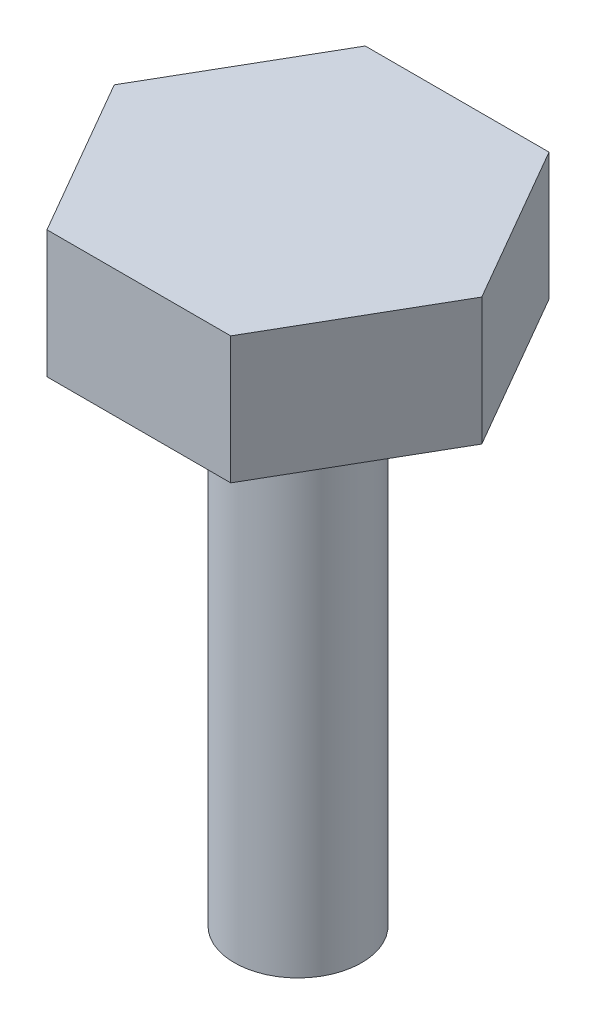
ISO-10303-21;
HEADER;
FILE_DESCRIPTION(('STEP AP214'),'2;1');
FILE_NAME('part.step','',(''),(''),'','','');
FILE_SCHEMA(('AUTOMOTIVE_DESIGN { 1 0 10303 214 1 1 1 1 }'));
ENDSEC;
DATA;
#1=APPLICATION_CONTEXT('core data for automotive mechanical design processes');
#2=APPLICATION_PROTOCOL_DEFINITION('international standard','automotive_design',2000,#1);
#3=PRODUCT_CONTEXT('',#1,'mechanical');
#4=PRODUCT('Part','Part','',(#3));
#5=PRODUCT_RELATED_PRODUCT_CATEGORY('part','',(#4));
#6=PRODUCT_DEFINITION_FORMATION('','',#4);
#7=PRODUCT_DEFINITION_CONTEXT('part definition',#1,'design');
#8=PRODUCT_DEFINITION('design','',#6,#7);
#9=PRODUCT_DEFINITION_SHAPE('','',#8);
#10=(LENGTH_UNIT() NAMED_UNIT(*) SI_UNIT(.MILLI.,.METRE.));
#11=(NAMED_UNIT(*) PLANE_ANGLE_UNIT() SI_UNIT($,.RADIAN.));
#12=(NAMED_UNIT(*) SI_UNIT($,.STERADIAN.) SOLID_ANGLE_UNIT());
#13=UNCERTAINTY_MEASURE_WITH_UNIT(LENGTH_MEASURE(1.E-05),#10,'distance_accuracy_value','');
#14=(GEOMETRIC_REPRESENTATION_CONTEXT(3) GLOBAL_UNCERTAINTY_ASSIGNED_CONTEXT((#13)) GLOBAL_UNIT_ASSIGNED_CONTEXT((#10,
#11,#12)) REPRESENTATION_CONTEXT('',''));
#15=CARTESIAN_POINT('',(0.,0.,0.));
#16=DIRECTION('',(0.,0.,1.));
#17=DIRECTION('',(1.,0.,0.));
#18=AXIS2_PLACEMENT_3D('',#15,#16,#17);
#19=CARTESIAN_POINT('',(14.4337567297409,20.,24.9999999999998));
#20=DIRECTION('',(-0.866025403784442,0.,-0.499999999999995));
#21=DIRECTION('',(-0.499999999999995,0.,0.866025403784442));
#22=AXIS2_PLACEMENT_3D('',#19,#20,#21);
#23=PLANE('',#22);
#24=DIRECTION('',(0.499999999999995,0.,-0.866025403784441));
#25=VECTOR('',#24,1.);
#26=CARTESIAN_POINT('',(14.4337567297409,0.,24.9999999999998));
#27=LINE('',#26,#25);
#28=CARTESIAN_POINT('',(14.4337567297409,0.,24.9999999999998));
#29=VERTEX_POINT('',#28);
#30=CARTESIAN_POINT('',(28.8675134594813,0.,0.));
#31=VERTEX_POINT('',#30);
#32=EDGE_CURVE('E124',#29,#31,#27,.T.);
#33=ORIENTED_EDGE('',*,*,#32,.T.);
#34=DIRECTION('',(0.,-1.,0.));
#35=VECTOR('',#34,1.);
#36=CARTESIAN_POINT('',(28.8675134594813,20.,0.));
#37=LINE('',#36,#35);
#38=CARTESIAN_POINT('',(28.8675134594813,20.,0.));
#39=VERTEX_POINT('',#38);
#40=EDGE_CURVE('E45',#39,#31,#37,.T.);
#41=ORIENTED_EDGE('',*,*,#40,.F.);
#42=DIRECTION('',(0.499999999999995,0.,-0.866025403784441));
#43=VECTOR('',#42,1.);
#44=CARTESIAN_POINT('',(14.4337567297409,20.,24.9999999999998));
#45=LINE('',#44,#43);
#46=CARTESIAN_POINT('',(14.4337567297409,20.,24.9999999999998));
#47=VERTEX_POINT('',#46);
#48=EDGE_CURVE('E138',#47,#39,#45,.T.);
#49=ORIENTED_EDGE('',*,*,#48,.F.);
#50=DIRECTION('',(0.,-1.,0.));
#51=VECTOR('',#50,1.);
#52=CARTESIAN_POINT('',(14.4337567297409,20.,24.9999999999998));
#53=LINE('',#52,#51);
#54=EDGE_CURVE('E123',#47,#29,#53,.T.);
#55=ORIENTED_EDGE('',*,*,#54,.T.);
#56=EDGE_LOOP('',(#33,#41,#49,#55));
#57=FACE_BOUND('',#56,.T.);
#58=ADVANCED_FACE('F39',(#57),#23,.F.);
#59=CARTESIAN_POINT('',(28.8675134594813,20.,0.));
#60=DIRECTION('',(-0.866025403784438,0.,0.500000000000001));
#61=DIRECTION('',(0.500000000000001,0.,0.866025403784438));
#62=AXIS2_PLACEMENT_3D('',#59,#60,#61);
#63=PLANE('',#62);
#64=DIRECTION('',(-0.500000000000001,0.,-0.866025403784438));
#65=VECTOR('',#64,1.);
#66=CARTESIAN_POINT('',(28.8675134594813,0.,0.));
#67=LINE('',#66,#65);
#68=CARTESIAN_POINT('',(14.4337567297406,0.,-25.0000000000001));
#69=VERTEX_POINT('',#68);
#70=EDGE_CURVE('E126',#31,#69,#67,.T.);
#71=ORIENTED_EDGE('',*,*,#70,.T.);
#72=DIRECTION('',(0.,-1.,0.));
#73=VECTOR('',#72,1.);
#74=CARTESIAN_POINT('',(14.4337567297406,20.,-25.0000000000001));
#75=LINE('',#74,#73);
#76=CARTESIAN_POINT('',(14.4337567297406,20.,-25.0000000000001));
#77=VERTEX_POINT('',#76);
#78=EDGE_CURVE('E137',#77,#69,#75,.T.);
#79=ORIENTED_EDGE('',*,*,#78,.F.);
#80=DIRECTION('',(-0.500000000000001,0.,-0.866025403784438));
#81=VECTOR('',#80,1.);
#82=CARTESIAN_POINT('',(28.8675134594813,20.,0.));
#83=LINE('',#82,#81);
#84=EDGE_CURVE('E94',#39,#77,#83,.T.);
#85=ORIENTED_EDGE('',*,*,#84,.F.);
#86=ORIENTED_EDGE('',*,*,#40,.T.);
#87=EDGE_LOOP('',(#71,#79,#85,#86));
#88=FACE_BOUND('',#87,.T.);
#89=ADVANCED_FACE('F145',(#88),#63,.F.);
#90=CARTESIAN_POINT('',(14.4337567297406,20.,-25.0000000000001));
#91=DIRECTION('',(0.,0.,1.));
#92=DIRECTION('',(1.,0.,0.));
#93=AXIS2_PLACEMENT_3D('',#90,#91,#92);
#94=PLANE('',#93);
#95=DIRECTION('',(-1.,0.,0.));
#96=VECTOR('',#95,1.);
#97=CARTESIAN_POINT('',(14.4337567297406,0.,-25.0000000000001));
#98=LINE('',#97,#96);
#99=CARTESIAN_POINT('',(-14.4337567297408,0.,-25.));
#100=VERTEX_POINT('',#99);
#101=EDGE_CURVE('E133',#69,#100,#98,.T.);
#102=ORIENTED_EDGE('',*,*,#101,.T.);
#103=DIRECTION('',(0.,-1.,0.));
#104=VECTOR('',#103,1.);
#105=CARTESIAN_POINT('',(-14.4337567297408,20.,-25.));
#106=LINE('',#105,#104);
#107=CARTESIAN_POINT('',(-14.4337567297408,20.,-25.));
#108=VERTEX_POINT('',#107);
#109=EDGE_CURVE('E118',#108,#100,#106,.T.);
#110=ORIENTED_EDGE('',*,*,#109,.F.);
#111=DIRECTION('',(-1.,0.,0.));
#112=VECTOR('',#111,1.);
#113=CARTESIAN_POINT('',(14.4337567297406,20.,-25.0000000000001));
#114=LINE('',#113,#112);
#115=EDGE_CURVE('E110',#77,#108,#114,.T.);
#116=ORIENTED_EDGE('',*,*,#115,.F.);
#117=ORIENTED_EDGE('',*,*,#78,.T.);
#118=EDGE_LOOP('',(#102,#110,#116,#117));
#119=FACE_BOUND('',#118,.T.);
#120=ADVANCED_FACE('F147',(#119),#94,.F.);
#121=CARTESIAN_POINT('',(-14.4337567297408,20.,-25.));
#122=DIRECTION('',(0.866025403784442,0.,0.499999999999995));
#123=DIRECTION('',(0.499999999999995,0.,-0.866025403784442));
#124=AXIS2_PLACEMENT_3D('',#121,#122,#123);
#125=PLANE('',#124);
#126=DIRECTION('',(-0.499999999999995,0.,0.866025403784442));
#127=VECTOR('',#126,1.);
#128=CARTESIAN_POINT('',(-14.4337567297408,0.,-25.));
#129=LINE('',#128,#127);
#130=CARTESIAN_POINT('',(-28.8675134594813,0.,2.01580769085164E-13));
#131=VERTEX_POINT('',#130);
#132=EDGE_CURVE('E113',#100,#131,#129,.T.);
#133=ORIENTED_EDGE('',*,*,#132,.T.);
#134=DIRECTION('',(0.,-1.,0.));
#135=VECTOR('',#134,1.);
#136=CARTESIAN_POINT('',(-28.8675134594813,20.,2.01580769085164E-13));
#137=LINE('',#136,#135);
#138=CARTESIAN_POINT('',(-28.8675134594813,20.,2.01580769085164E-13));
#139=VERTEX_POINT('',#138);
#140=EDGE_CURVE('E115',#139,#131,#137,.T.);
#141=ORIENTED_EDGE('',*,*,#140,.F.);
#142=DIRECTION('',(-0.499999999999995,0.,0.866025403784442));
#143=VECTOR('',#142,1.);
#144=CARTESIAN_POINT('',(-14.4337567297408,20.,-25.));
#145=LINE('',#144,#143);
#146=EDGE_CURVE('E101',#108,#139,#145,.T.);
#147=ORIENTED_EDGE('',*,*,#146,.F.);
#148=ORIENTED_EDGE('',*,*,#109,.T.);
#149=EDGE_LOOP('',(#133,#141,#147,#148));
#150=FACE_BOUND('',#149,.T.);
#151=ADVANCED_FACE('F114',(#150),#125,.F.);
#152=CARTESIAN_POINT('',(-28.8675134594813,20.,2.01580769085164E-13));
#153=DIRECTION('',(0.866025403784435,0.,-0.500000000000007));
#154=DIRECTION('',(-0.500000000000007,0.,-0.866025403784435));
#155=AXIS2_PLACEMENT_3D('',#152,#153,#154);
#156=PLANE('',#155);
#157=DIRECTION('',(0.500000000000007,0.,0.866025403784435));
#158=VECTOR('',#157,1.);
#159=CARTESIAN_POINT('',(-28.8675134594813,0.,2.01580769085164E-13));
#160=LINE('',#159,#158);
#161=CARTESIAN_POINT('',(-14.4337567297404,0.,25.0000000000001));
#162=VERTEX_POINT('',#161);
#163=EDGE_CURVE('E77',#131,#162,#160,.T.);
#164=ORIENTED_EDGE('',*,*,#163,.T.);
#165=DIRECTION('',(0.,-1.,0.));
#166=VECTOR('',#165,1.);
#167=CARTESIAN_POINT('',(-14.4337567297404,20.,25.0000000000001));
#168=LINE('',#167,#166);
#169=CARTESIAN_POINT('',(-14.4337567297404,20.,25.0000000000001));
#170=VERTEX_POINT('',#169);
#171=EDGE_CURVE('E120',#170,#162,#168,.T.);
#172=ORIENTED_EDGE('',*,*,#171,.F.);
#173=DIRECTION('',(0.500000000000007,0.,0.866025403784435));
#174=VECTOR('',#173,1.);
#175=CARTESIAN_POINT('',(-28.8675134594813,20.,2.01580769085164E-13));
#176=LINE('',#175,#174);
#177=EDGE_CURVE('E104',#139,#170,#176,.T.);
#178=ORIENTED_EDGE('',*,*,#177,.F.);
#179=ORIENTED_EDGE('',*,*,#140,.T.);
#180=EDGE_LOOP('',(#164,#172,#178,#179));
#181=FACE_BOUND('',#180,.T.);
#182=ADVANCED_FACE('F117',(#181),#156,.F.);
#183=CARTESIAN_POINT('',(-14.4337567297404,20.,25.0000000000001));
#184=DIRECTION('',(0.,0.,-1.));
#185=DIRECTION('',(-1.,0.,0.));
#186=AXIS2_PLACEMENT_3D('',#183,#184,#185);
#187=PLANE('',#186);
#188=DIRECTION('',(1.,0.,0.));
#189=VECTOR('',#188,1.);
#190=CARTESIAN_POINT('',(-14.4337567297404,0.,25.0000000000001));
#191=LINE('',#190,#189);
#192=EDGE_CURVE('E84',#162,#29,#191,.T.);
#193=ORIENTED_EDGE('',*,*,#192,.T.);
#194=ORIENTED_EDGE('',*,*,#54,.F.);
#195=DIRECTION('',(1.,0.,0.));
#196=VECTOR('',#195,1.);
#197=CARTESIAN_POINT('',(-14.4337567297404,20.,25.0000000000001));
#198=LINE('',#197,#196);
#199=EDGE_CURVE('E57',#170,#47,#198,.T.);
#200=ORIENTED_EDGE('',*,*,#199,.F.);
#201=ORIENTED_EDGE('',*,*,#171,.T.);
#202=EDGE_LOOP('',(#193,#194,#200,#201));
#203=FACE_BOUND('',#202,.T.);
#204=ADVANCED_FACE('F168',(#203),#187,.F.);
#205=CARTESIAN_POINT('',(0.,20.,0.));
#206=DIRECTION('',(0.,1.,0.));
#207=DIRECTION('',(0.,0.,1.));
#208=AXIS2_PLACEMENT_3D('',#205,#206,#207);
#209=PLANE('',#208);
#210=ORIENTED_EDGE('',*,*,#48,.T.);
#211=ORIENTED_EDGE('',*,*,#84,.T.);
#212=ORIENTED_EDGE('',*,*,#115,.T.);
#213=ORIENTED_EDGE('',*,*,#146,.T.);
#214=ORIENTED_EDGE('',*,*,#177,.T.);
#215=ORIENTED_EDGE('',*,*,#199,.T.);
#216=EDGE_LOOP('',(#210,#211,#212,#213,#214,#215));
#217=FACE_BOUND('',#216,.T.);
#218=ADVANCED_FACE('F103',(#217),#209,.T.);
#219=CARTESIAN_POINT('',(0.,0.,0.));
#220=DIRECTION('',(0.,1.,0.));
#221=DIRECTION('',(0.,0.,1.));
#222=AXIS2_PLACEMENT_3D('',#219,#220,#221);
#223=PLANE('',#222);
#224=CARTESIAN_POINT('',(0.,0.,0.));
#225=DIRECTION('',(0.,-1.,0.));
#226=DIRECTION('',(0.,0.,-1.));
#227=AXIS2_PLACEMENT_3D('',#224,#225,#226);
#228=CIRCLE('',#227,10.);
#229=CARTESIAN_POINT('',(0.,0.,-10.));
#230=VERTEX_POINT('',#229);
#231=EDGE_CURVE('E11',#230,#230,#228,.T.);
#232=ORIENTED_EDGE('',*,*,#231,.F.);
#233=EDGE_LOOP('',(#232));
#234=FACE_BOUND('',#233,.T.);
#235=ORIENTED_EDGE('',*,*,#32,.F.);
#236=ORIENTED_EDGE('',*,*,#192,.F.);
#237=ORIENTED_EDGE('',*,*,#163,.F.);
#238=ORIENTED_EDGE('',*,*,#132,.F.);
#239=ORIENTED_EDGE('',*,*,#101,.F.);
#240=ORIENTED_EDGE('',*,*,#70,.F.);
#241=EDGE_LOOP('',(#235,#236,#237,#238,#239,#240));
#242=FACE_BOUND('',#241,.T.);
#243=ADVANCED_FACE('F149',(#234,#242),#223,.F.);
#244=CARTESIAN_POINT('',(0.,-80.,0.));
#245=DIRECTION('',(0.,1.,0.));
#246=DIRECTION('',(0.,0.,1.));
#247=AXIS2_PLACEMENT_3D('',#244,#245,#246);
#248=CYLINDRICAL_SURFACE('',#247,10.);
#249=CARTESIAN_POINT('',(0.,-80.,0.));
#250=DIRECTION('',(0.,-1.,0.));
#251=DIRECTION('',(0.,0.,-1.));
#252=AXIS2_PLACEMENT_3D('',#249,#250,#251);
#253=CIRCLE('',#252,10.);
#254=CARTESIAN_POINT('',(0.,-80.,-10.));
#255=VERTEX_POINT('',#254);
#256=EDGE_CURVE('E129',#255,#255,#253,.T.);
#257=ORIENTED_EDGE('',*,*,#256,.F.);
#258=EDGE_LOOP('',(#257));
#259=FACE_BOUND('',#258,.T.);
#260=ORIENTED_EDGE('',*,*,#231,.T.);
#261=EDGE_LOOP('',(#260));
#262=FACE_BOUND('',#261,.T.);
#263=ADVANCED_FACE('F157',(#259,#262),#248,.T.);
#264=CARTESIAN_POINT('',(0.,-80.,0.));
#265=DIRECTION('',(0.,-1.,0.));
#266=DIRECTION('',(0.,0.,-1.));
#267=AXIS2_PLACEMENT_3D('',#264,#265,#266);
#268=PLANE('',#267);
#269=ORIENTED_EDGE('',*,*,#256,.T.);
#270=EDGE_LOOP('',(#269));
#271=FACE_BOUND('',#270,.T.);
#272=ADVANCED_FACE('F160',(#271),#268,.T.);
#273=CLOSED_SHELL('',(#58,#89,#120,#151,#182,#204,#218,#243,#263,#272));
#274=MANIFOLD_SOLID_BREP('B2',#273);
#275=ADVANCED_BREP_SHAPE_REPRESENTATION('',(#18,#274),#14);
#276=SHAPE_DEFINITION_REPRESENTATION(#9,#275);
ENDSEC;
END-ISO-10303-21;
